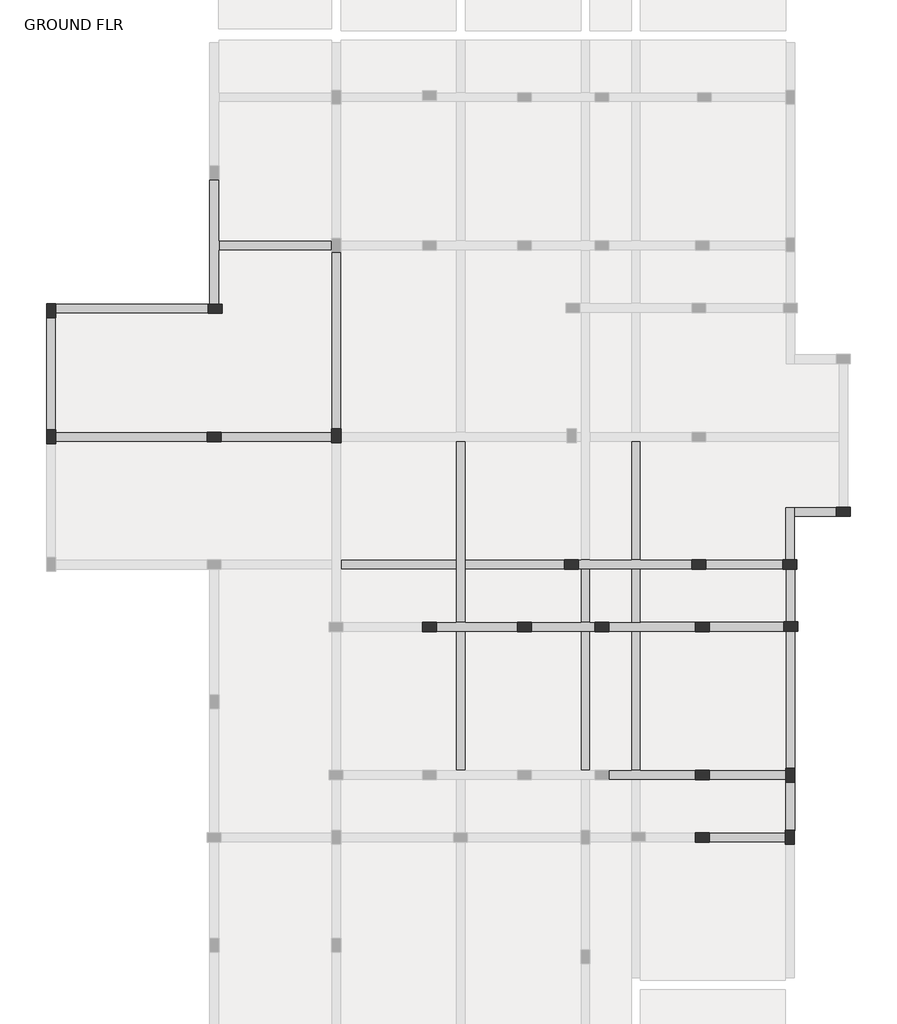
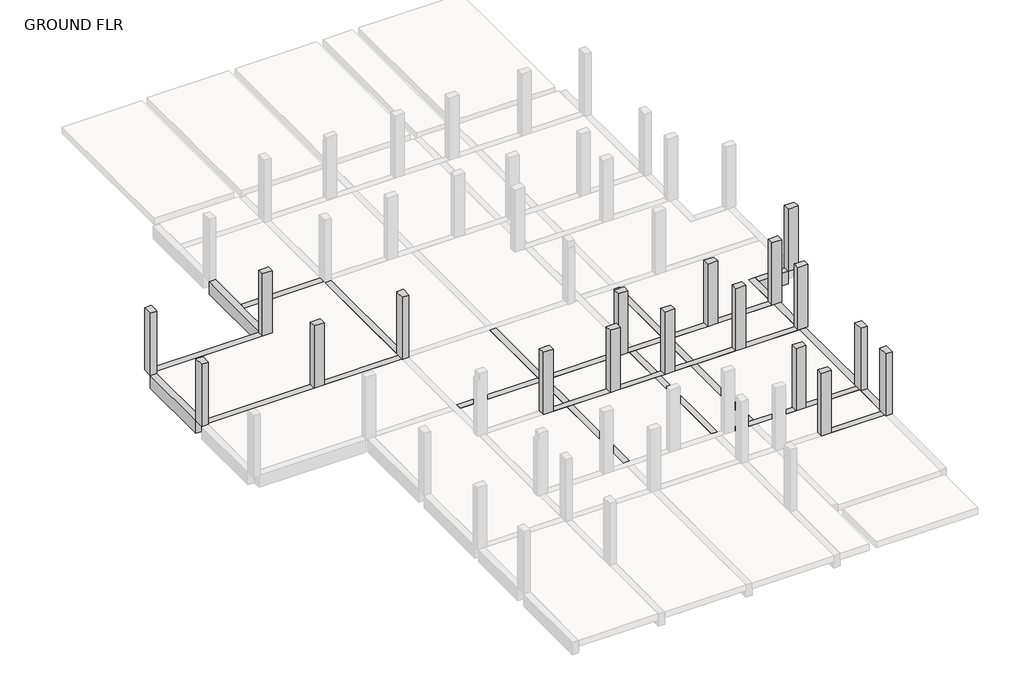
# One storey, part 3 of 5: 30 beams, 18 columns.
"""IFC4 building model written with IfcOpenShell, lengths in millimetres."""

from ifc_helpers import new_model, si_unit, frame, origin, place, context, project, spatial, polyline, outline, extrude, faceted_brep, element, save

model = new_model("IFC4")

# Units and contexts
model_context = context("Model", 3, world=origin())
ifc_project = project(units=[si_unit("LENGTHUNIT", "METRE", prefix="MILLI")], contexts=[model_context])

# Site, building, storey
site = spatial("IfcSite", under=ifc_project)
building = spatial("IfcBuilding", under=site)
storey = spatial("IfcBuildingStorey", under=building, Name="GROUND FLR", Elevation=0.0)

# Beams
placement = place(None, origin())
element("IfcBeam", 1, ObjectType="M_Concrete-Rectangular Beam : 300 x 600mm", at=placement, inside=storey, context=model_context, shape_type="Brep", body=[
    faceted_brep([(-5888.8105653, 9367.5252033, 0.0), (-5888.8105653, 5367.5252033, 0.0), (-5588.8105653, 5367.5252033, 0.0), (-5588.8105653, 7099.7076276, 0.0), (-5588.8105653, 7399.7076276, 0.0), (-5588.8105653, 9367.5252033, 0.0), (-5888.8105653, 9367.5252033, -600.0), (-5888.8105653, 5367.5252033, -600.0), (-5588.8105653, 9367.5252033, -600.0), (-5588.8105653, 7399.7076276, -600.0), (-5588.8105653, 7099.7076276, -600.0), (-5588.8105653, 5367.5252033, -600.0), (-5588.8105653, 9367.5252033, -300.0), (-5588.8105653, 5367.5252033, -300.0)], [[[0, 1, 2, 3, 4, 5]], [[1, 0, 6, 7]], [[7, 6, 8, 9, 10, 11]], [[11, 10, 9, 8, 12, 5, 4, 3, 2, 13]], [[8, 6, 0, 5, 12]], [[2, 1, 7, 11, 13]]]),
])
element("IfcBeam", 2, ObjectType="M_Concrete-Rectangular Beam : 300 x 600mm", at=placement, inside=storey, context=model_context, shape_type="Brep", body=[
    faceted_brep([(-5943.8105653, 5067.6057249, 0.0), (-5943.8105653, 5367.6057249, 0.0), (-10828.8105653, 5367.6057249, 0.0), (-10828.8105653, 5067.6057249, 0.0), (-5943.8105653, 5367.6057249, -600.0), (-10828.8105653, 5367.6057249, -600.0), (-5943.8105653, 5067.6057249, -600.0), (-10828.8105653, 5067.6057249, -600.0), (-10828.8105653, 5067.6057249, -300.0), (-5943.8105653, 5067.6057249, -300.0)], [[[0, 1, 2, 3]], [[1, 4, 5, 2]], [[4, 6, 7, 5]], [[0, 3, 8, 7, 6, 9]], [[6, 4, 1, 0, 9]], [[3, 2, 5, 7, 8]]]),
])
element("IfcBeam", 3, ObjectType="M_Concrete-Rectangular Beam : 300 x 600mm", at=placement, inside=storey, context=model_context, shape_type="SweptSolid", body=[
    extrude(outline(polyline([(-10828.8105653, 1326.1713929), (-11128.8105653, 1326.1713929), (-11128.8105653, 4932.6057249), (-10828.8105653, 4932.6057249), (-10828.8105653, 1326.1713929)])), frame((0.0, 0.0, -600.0), z_axis=(0.0, 0.0, 1.0), x_axis=(1.0, 0.0, 0.0)), (0.0, 0.0, 1.0), 600.0),
])
element("IfcBeam", 4, ObjectType="M_Concrete-Rectangular Beam : 300 x 600mm", at=placement, inside=storey, context=model_context, shape_type="SweptSolid", body=[
    extrude(outline(polyline([(12619.1163908, -9982.1078267), (12919.1163908, -9982.1078267), (12919.1163908, -11537.8970059), (12899.1163908, -11537.8970059), (12899.1163908, -11532.8970059), (12619.1163908, -11532.8970059), (12619.1163908, -9982.1078267)])), frame((0.0, 0.0, -600.0), z_axis=(0.0, 0.0, 1.0), x_axis=(1.0, 0.0, 0.0)), (0.0, 0.0, 1.0), 600.0),
])
element("IfcBeam", 5, ObjectType="M_Concrete-Rectangular Beam : 300 x 600mm", at=placement, inside=storey, context=model_context, shape_type="Brep", body=[
    faceted_brep([(12619.1163908, -5144.3229916, 0.0), (12919.1163908, -5144.3229916, 0.0), (12919.1163908, -5144.3229916, -600.0), (12619.1163908, -5144.3229916, -600.0), (12619.1163908, -5151.6229916, 0.0), (12619.1163908, -9532.1078267, 0.0), (12919.1163908, -9532.1078267, 0.0), (12919.1163908, -9532.1078267, -600.0), (12619.1163908, -9532.1078267, -600.0), (12619.1163908, -5151.6229916, -600.0), (12619.1163908, -9532.1078267, -300.0)], [[[0, 1, 2, 3]], [[1, 0, 4, 5, 6]], [[2, 1, 6, 7]], [[3, 2, 7, 8, 9]], [[0, 3, 9, 8, 10, 5, 4]], [[8, 7, 6, 5, 10]]]),
])
element("IfcBeam", 6, ObjectType="M_Concrete-Rectangular Beam : 300 x 600mm", at=placement, inside=storey, context=model_context, shape_type="Brep", body=[
    faceted_brep([(12619.1163908, -4818.9229916, -600.0), (12919.1163908, -4818.9229916, -600.0), (12919.1163908, -4818.9229916, 0.0), (12619.1163908, -4818.9229916, 0.0), (12619.1163908, -4818.9229916, -300.0), (12919.1163908, -3139.4535766, 0.0), (12619.1163908, -3139.4535766, 0.0), (12919.1163908, -3139.4535766, -600.0), (12619.1163908, -3139.4535766, -600.0), (12619.1163908, -3139.4535766, -300.0)], [[[0, 1, 2, 3, 4]], [[3, 2, 5, 6]], [[2, 1, 7, 5]], [[1, 0, 8, 7]], [[3, 6, 9, 8, 0, 4]], [[6, 5, 7, 8, 9]]]),
])
element("IfcBeam", 7, ObjectType="M_Concrete-Rectangular Beam : 300 x 600mm", at=placement, inside=storey, context=model_context, shape_type="Brep", body=[
    faceted_brep([(12599.1163908, -2839.4535766, 0.0), (12899.1163908, -2839.4535766, 0.0), (12899.1163908, -1448.8286071, 0.0), (12899.1163908, -1148.8286071, 0.0), (12599.1163908, -1148.8286071, 0.0), (12899.1163908, -2839.4535766, -600.0), (12899.1163908, -1448.8286071, -600.0), (12899.1163908, -1148.8286071, -600.0), (12899.1163908, -1148.8286071, -300.0), (12599.1163908, -2839.4535766, -600.0), (12599.1163908, -1148.8286071, -600.0), (12599.1163908, -1148.8286071, -300.0), (12599.1163908, -2839.4535766, -300.0)], [[[0, 1, 2, 3, 4]], [[1, 5, 6, 7, 8, 3, 2]], [[5, 9, 10, 7, 6]], [[0, 4, 11, 10, 9, 12]], [[9, 5, 1, 0, 12]], [[4, 3, 8, 7, 10, 11]]]),
])
element("IfcBeam", 8, ObjectType="M_Concrete-Rectangular Beam : 300 x 600mm", at=placement, inside=storey, context=model_context, shape_type="Brep", body=[
    faceted_brep([(14244.1163908, -1448.8286071, 0.0), (14244.1163908, -1148.8286071, 0.0), (12899.1163908, -1148.8286071, 0.0), (12899.1163908, -1448.8286071, 0.0), (14244.1163908, -1148.8286071, -300.0), (14244.1163908, -1148.8286071, -600.0), (12899.1163908, -1148.8286071, -600.0), (12899.1163908, -1148.8286071, -300.0), (14244.1163908, -1448.8286071, -600.0), (12899.1163908, -1448.8286071, -600.0)], [[[0, 1, 2, 3]], [[2, 1, 4, 5, 6, 7]], [[5, 8, 9, 6]], [[8, 0, 3, 9]], [[0, 8, 5, 4, 1]], [[3, 2, 7, 6, 9]]]),
])
element("IfcBeam", 9, ObjectType="M_Concrete-Rectangular Beam : 300 x 600mm", at=placement, inside=storey, context=model_context, shape_type="Brep", body=[
    faceted_brep([(-1671.7865686, 7024.7076276, 0.0), (-1971.7865686, 7024.7076276, 0.0), (-1971.7865686, 1366.1713929, 0.0), (-1671.7865686, 1366.1713929, 0.0), (-1971.7865686, 7024.7076276, -300.0), (-1971.7865686, 7024.7076276, -600.0), (-1971.7865686, 1366.1713929, -600.0), (-1971.7865686, 1366.1713929, -300.0), (-1671.7865686, 7024.7076276, -600.0), (-1671.7865686, 1366.1713929, -600.0), (-1671.7865686, 1366.1713929, -300.0), (-1671.7865686, 7024.7076276, -300.0)], [[[0, 1, 2, 3]], [[2, 1, 4, 5, 6, 7]], [[5, 8, 9, 6]], [[0, 3, 10, 9, 8, 11]], [[1, 0, 11, 8, 5, 4]], [[3, 2, 7, 6, 9, 10]]]),
])
element("IfcBeam", 10, ObjectType="M_Concrete-Rectangular Beam : 300 x 600mm", at=placement, inside=storey, context=model_context, shape_type="Brep", body=[
    faceted_brep([(-1971.7865686, 7099.7076276, 0.0), (-1971.7865686, 7399.7076276, 0.0), (-5588.8105653, 7399.7076276, 0.0), (-5588.8105653, 7099.7076276, 0.0), (-5588.8105653, 7099.7076276, -300.0), (-5588.8105653, 7099.7076276, -600.0), (-1971.7865686, 7099.7076276, -600.0), (-1971.7865686, 7099.7076276, -300.0), (-1971.7865686, 7399.7076276, -600.0), (-5588.8105653, 7399.7076276, -600.0), (-1971.7865686, 7399.7076276, -300.0), (-5588.8105653, 7399.7076276, -300.0)], [[[0, 1, 2, 3]], [[0, 3, 4, 5, 6, 7]], [[8, 6, 5, 9]], [[2, 1, 10, 8, 9, 11]], [[1, 0, 7, 6, 8, 10]], [[3, 2, 11, 9, 5, 4]]]),
])
element("IfcBeam", 11, ObjectType="M_Concrete-Rectangular Beam : 300 x 600mm", at=placement, inside=storey, context=model_context, shape_type="Brep", body=[
    faceted_brep([(-10828.8105653, 1251.1713929, 0.0), (-10828.8105653, 951.1713929, 0.0), (-5963.8105653, 951.1713929, 0.0), (-5963.8105653, 1251.1713929, 0.0), (-10828.8105653, 951.1713929, -300.0), (-10828.8105653, 951.1713929, -600.0), (-5963.8105653, 951.1713929, -600.0), (-5963.8105653, 951.1713929, -300.0), (-10828.8105653, 1251.1713929, -600.0), (-5963.8105653, 1251.1713929, -600.0), (-5963.8105653, 1251.1713929, -300.0), (-10828.8105653, 1251.1713929, -300.0)], [[[0, 1, 2, 3]], [[2, 1, 4, 5, 6, 7]], [[5, 8, 9, 6]], [[0, 3, 10, 9, 8, 11]], [[1, 0, 11, 8, 5, 4]], [[3, 2, 7, 6, 9, 10]]]),
])
element("IfcBeam", 12, ObjectType="M_Concrete-Rectangular Beam : 300 x 600mm", at=placement, inside=storey, context=model_context, shape_type="Brep", body=[
    faceted_brep([(-5513.8105653, 1251.1713929, 0.0), (-5513.8105653, 951.1713929, 0.0), (-1971.7865686, 951.1713929, 0.0), (-1971.7865686, 1251.1713929, 0.0), (-5513.8105653, 951.1713929, -300.0), (-5513.8105653, 951.1713929, -600.0), (-1971.7865686, 951.1713929, -600.0), (-1971.7865686, 951.1713929, -300.0), (-5513.8105653, 1251.1713929, -600.0), (-1971.7865686, 1251.1713929, -600.0), (-1971.7865686, 1251.1713929, -300.0), (-5513.8105653, 1251.1713929, -300.0)], [[[0, 1, 2, 3]], [[2, 1, 4, 5, 6, 7]], [[5, 8, 9, 6]], [[0, 3, 10, 9, 8, 11]], [[1, 0, 11, 8, 5, 4]], [[3, 2, 7, 6, 9, 10]]]),
])
element("IfcBeam", 13, ObjectType="M_Concrete-Rectangular Beam : 300 x 600mm", at=placement, inside=storey, context=model_context, shape_type="Brep", body=[
    faceted_brep([(9601.8679014, -3139.4535766, 0.0), (9601.8679014, -2839.4535766, 0.0), (7956.8679014, -2839.4535766, 0.0), (7656.8679014, -2839.4535766, 0.0), (6332.5248054, -2839.4535766, 0.0), (6032.5248054, -2839.4535766, 0.0), (5967.5248054, -2839.4535766, 0.0), (5967.5248054, -3139.4535766, 0.0), (6032.5248054, -3139.4535766, 0.0), (6332.5248054, -3139.4535766, 0.0), (7656.8679014, -3139.4535766, 0.0), (7956.8679014, -3139.4535766, 0.0), (5967.5248054, -3139.4535766, -600.0), (6032.5248054, -3139.4535766, -600.0), (6332.5248054, -3139.4535766, -600.0), (7656.8679014, -3139.4535766, -600.0), (7956.8679014, -3139.4535766, -600.0), (9601.8679014, -3139.4535766, -600.0), (9601.8679014, -3139.4535766, -300.0), (5967.5248054, -3139.4535766, -300.0), (9601.8679014, -2839.4535766, -600.0), (5967.5248054, -2839.4535766, -600.0), (6032.5248054, -2839.4535766, -600.0), (6332.5248054, -2839.4535766, -600.0), (7656.8679014, -2839.4535766, -600.0), (7956.8679014, -2839.4535766, -600.0), (5967.5248054, -2839.4535766, -300.0), (9601.8679014, -2839.4535766, -300.0)], [[[0, 1, 2, 3, 4, 5, 6, 7, 8, 9, 10, 11]], [[12, 13, 14, 15, 16, 17, 18, 0, 11, 10, 9, 8, 7, 19]], [[20, 17, 16, 15, 14, 13, 12, 21, 22, 23, 24, 25]], [[20, 25, 24, 23, 22, 21, 26, 6, 5, 4, 3, 2, 1, 27]], [[1, 0, 18, 17, 20, 27]], [[7, 6, 26, 21, 12, 19]]]),
])
element("IfcBeam", 14, ObjectType="M_Concrete-Rectangular Beam : 300 x 600mm", at=placement, inside=storey, context=model_context, shape_type="Brep", body=[
    faceted_brep([(12524.1163908, -3139.4535766, 0.0), (12524.1163908, -2839.4535766, 0.0), (10051.8679014, -2839.4535766, 0.0), (10051.8679014, -3139.4535766, 0.0), (10051.8679014, -3139.4535766, -300.0), (10051.8679014, -3139.4535766, -600.0), (12524.1163908, -3139.4535766, -600.0), (12524.1163908, -3139.4535766, -300.0), (12524.1163908, -2839.4535766, -600.0), (10051.8679014, -2839.4535766, -600.0), (12524.1163908, -2839.4535766, -300.0), (10051.8679014, -2839.4535766, -300.0)], [[[0, 1, 2, 3]], [[0, 3, 4, 5, 6, 7]], [[8, 6, 5, 9]], [[2, 1, 10, 8, 9, 11]], [[1, 0, 7, 6, 8, 10]], [[3, 2, 11, 9, 5, 4]]]),
])
element("IfcBeam", 15, ObjectType="M_Concrete-Rectangular Beam : 300 x 600mm", at=placement, inside=storey, context=model_context, shape_type="Brep", body=[
    faceted_brep([(1399.7296816, -4851.6229916, 0.0), (1399.7296816, -5151.6229916, 0.0), (2024.7296816, -5151.6229916, 0.0), (2324.7296816, -5151.6229916, 0.0), (3997.5248054, -5151.6229916, 0.0), (3997.5248054, -4851.6229916, 0.0), (2324.7296816, -4851.6229916, 0.0), (2024.7296816, -4851.6229916, 0.0), (1399.7296816, -5151.6229916, -600.0), (2024.7296816, -5151.6229916, -600.0), (2324.7296816, -5151.6229916, -600.0), (3997.5248054, -5151.6229916, -600.0), (3997.5248054, -5151.6229916, -300.0), (1399.7296816, -5151.6229916, -300.0), (1399.7296816, -4851.6229916, -600.0), (2024.7296816, -4851.6229916, -600.0), (2324.7296816, -4851.6229916, -600.0), (3997.5248054, -4851.6229916, -600.0), (1399.7296816, -4851.6229916, -300.0), (3997.5248054, -4851.6229916, -300.0)], [[[0, 1, 2, 3, 4, 5, 6, 7]], [[8, 9, 10, 11, 12, 4, 3, 2, 1, 13]], [[8, 14, 15, 16, 17, 11, 10, 9]], [[17, 16, 15, 14, 18, 0, 7, 6, 5, 19]], [[1, 0, 18, 14, 8, 13]], [[5, 4, 12, 11, 17, 19]]]),
])
element("IfcBeam", 16, ObjectType="M_Concrete-Rectangular Beam : 300 x 600mm", at=placement, inside=storey, context=model_context, shape_type="Brep", body=[
    faceted_brep([(4447.5248054, -4851.6229916, 0.0), (4447.5248054, -5151.6229916, 0.0), (6032.5248054, -5151.6229916, 0.0), (6332.5248054, -5151.6229916, 0.0), (6481.8679014, -5151.6229916, 0.0), (6481.8679014, -4851.6229916, 0.0), (6332.5248054, -4851.6229916, 0.0), (6032.5248054, -4851.6229916, 0.0), (4447.5248054, -5151.6229916, -600.0), (6032.5248054, -5151.6229916, -600.0), (6332.5248054, -5151.6229916, -600.0), (6481.8679014, -5151.6229916, -600.0), (6481.8679014, -5151.6229916, -300.0), (4447.5248054, -5151.6229916, -300.0), (4447.5248054, -4851.6229916, -600.0), (6032.5248054, -4851.6229916, -600.0), (6332.5248054, -4851.6229916, -600.0), (6481.8679014, -4851.6229916, -600.0), (4447.5248054, -4851.6229916, -300.0)], [[[0, 1, 2, 3, 4, 5, 6, 7]], [[8, 9, 10, 11, 12, 4, 3, 2, 1, 13]], [[8, 14, 15, 16, 17, 11, 10, 9]], [[17, 16, 15, 14, 18, 0, 7, 6, 5]], [[1, 0, 18, 14, 8, 13]], [[5, 4, 12, 11, 17]]]),
])
element("IfcBeam", 17, ObjectType="M_Concrete-Rectangular Beam : 300 x 600mm", at=placement, inside=storey, context=model_context, shape_type="Brep", body=[
    faceted_brep([(6931.8679014, -4851.6229916, 0.0), (6931.8679014, -5151.6229916, 0.0), (7656.8679014, -5151.6229916, 0.0), (7956.8679014, -5151.6229916, 0.0), (9721.8679014, -5151.6229916, 0.0), (9721.8679014, -4851.6229916, 0.0), (7956.8679014, -4851.6229916, 0.0), (7656.8679014, -4851.6229916, 0.0), (6931.8679014, -5151.6229916, -600.0), (7656.8679014, -5151.6229916, -600.0), (7956.8679014, -5151.6229916, -600.0), (9721.8679014, -5151.6229916, -600.0), (9721.8679014, -5151.6229916, -300.0), (6931.8679014, -5151.6229916, -300.0), (6931.8679014, -4851.6229916, -600.0), (7656.8679014, -4851.6229916, -600.0), (7956.8679014, -4851.6229916, -600.0), (9721.8679014, -4851.6229916, -600.0)], [[[0, 1, 2, 3, 4, 5, 6, 7]], [[8, 9, 10, 11, 12, 4, 3, 2, 1, 13]], [[8, 14, 15, 16, 17, 11, 10, 9]], [[14, 0, 7, 6, 5, 17, 16, 15]], [[1, 0, 14, 8, 13]], [[5, 4, 12, 11, 17]]]),
])
element("IfcBeam", 18, ObjectType="M_Concrete-Rectangular Beam : 300 x 600mm", at=placement, inside=storey, context=model_context, shape_type="Brep", body=[
    faceted_brep([(12599.1163908, -11907.8970059, 0.0), (12599.1163908, -11607.8970059, 0.0), (10171.8679014, -11607.8970059, 0.0), (10171.8679014, -11907.8970059, 0.0), (10171.8679014, -11907.8970059, -300.0), (10171.8679014, -11907.8970059, -600.0), (12599.1163908, -11907.8970059, -600.0), (12599.1163908, -11907.8970059, -300.0), (12599.1163908, -11607.8970059, -600.0), (10171.8679014, -11607.8970059, -600.0), (12599.1163908, -11607.8970059, -300.0), (10171.8679014, -11607.8970059, -300.0)], [[[0, 1, 2, 3]], [[0, 3, 4, 5, 6, 7]], [[8, 6, 5, 9]], [[2, 1, 10, 8, 9, 11]], [[1, 0, 7, 6, 8, 10]], [[3, 2, 11, 9, 5, 4]]]),
])
element("IfcBeam", 19, ObjectType="M_Concrete-Rectangular Beam : 300 x 600mm", at=placement, inside=storey, context=model_context, shape_type="Brep", body=[
    faceted_brep([(6931.8679014, -9607.1078267, 0.0), (6931.8679014, -9907.1078267, 0.0), (7656.8679014, -9907.1078267, 0.0), (7956.8679014, -9907.1078267, 0.0), (9721.8679014, -9907.1078267, 0.0), (9721.8679014, -9607.1078267, 0.0), (7956.8679014, -9607.1078267, 0.0), (7656.8679014, -9607.1078267, 0.0), (6931.8679014, -9907.1078267, -600.0), (7656.8679014, -9907.1078267, -600.0), (7956.8679014, -9907.1078267, -600.0), (9721.8679014, -9907.1078267, -600.0), (9721.8679014, -9907.1078267, -300.0), (6931.8679014, -9907.1078267, -300.0), (6931.8679014, -9607.1078267, -600.0), (7656.8679014, -9607.1078267, -600.0), (7956.8679014, -9607.1078267, -600.0), (9721.8679014, -9607.1078267, -600.0), (6931.8679014, -9607.1078267, -300.0), (9721.8679014, -9607.1078267, -300.0)], [[[0, 1, 2, 3, 4, 5, 6, 7]], [[8, 9, 10, 11, 12, 4, 3, 2, 1, 13]], [[8, 14, 15, 16, 17, 11, 10, 9]], [[17, 16, 15, 14, 18, 0, 7, 6, 5, 19]], [[1, 0, 18, 14, 8, 13]], [[5, 4, 12, 11, 17, 19]]]),
])
element("IfcBeam", 20, ObjectType="M_Concrete-Rectangular Beam : 300 x 600mm", at=placement, inside=storey, context=model_context, shape_type="Brep", body=[
    faceted_brep([(10171.8679014, -9607.1078267, 0.0), (10171.8679014, -9907.1078267, 0.0), (12599.1163908, -9907.1078267, 0.0), (12619.1163908, -9907.1078267, 0.0), (12619.1163908, -9607.1078267, 0.0), (10171.8679014, -9907.1078267, -600.0), (12619.1163908, -9907.1078267, -600.0), (10171.8679014, -9907.1078267, -300.0), (10171.8679014, -9607.1078267, -600.0), (12619.1163908, -9607.1078267, -600.0), (12619.1163908, -9607.1078267, -300.0), (10171.8679014, -9607.1078267, -300.0)], [[[0, 1, 2, 3, 4]], [[5, 6, 3, 2, 1, 7]], [[5, 8, 9, 6]], [[0, 4, 10, 9, 8, 11]], [[1, 0, 11, 8, 5, 7]], [[4, 3, 6, 9, 10]]]),
])
element("IfcBeam", 21, ObjectType="M_Concrete-Rectangular Beam : 300 x 600mm", at=placement, inside=storey, context=model_context, shape_type="Brep", body=[
    faceted_brep([(-1671.7865686, -2839.4535766, 0.0), (-1671.7865686, -3139.4535766, 0.0), (2024.7296816, -3139.4535766, 0.0), (2024.7296816, -2839.4535766, 0.0), (-1671.7865686, -3139.4535766, -300.0), (-1671.7865686, -3139.4535766, -600.0), (2024.7296816, -3139.4535766, -600.0), (2024.7296816, -3139.4535766, -300.0), (-1671.7865686, -2839.4535766, -600.0), (2024.7296816, -2839.4535766, -600.0), (2024.7296816, -2839.4535766, -300.0), (-1671.7865686, -2839.4535766, -300.0)], [[[0, 1, 2, 3]], [[2, 1, 4, 5, 6, 7]], [[5, 8, 9, 6]], [[0, 3, 10, 9, 8, 11]], [[1, 0, 11, 8, 5, 4]], [[3, 2, 7, 6, 9, 10]]]),
])
element("IfcBeam", 22, ObjectType="M_Concrete-Rectangular Beam : 300 x 600mm", at=placement, inside=storey, context=model_context, shape_type="Brep", body=[
    faceted_brep([(6332.5248054, -3139.4535766, 0.0), (6032.5248054, -3139.4535766, 0.0), (6032.5248054, -4851.6229916, 0.0), (6332.5248054, -4851.6229916, 0.0), (6032.5248054, -3139.4535766, -300.0), (6032.5248054, -3139.4535766, -600.0), (6032.5248054, -4851.6229916, -600.0), (6032.5248054, -4851.6229916, -300.0), (6332.5248054, -3139.4535766, -600.0), (6332.5248054, -4851.6229916, -600.0), (6332.5248054, -3139.4535766, -300.0), (6332.5248054, -4851.6229916, -300.0)], [[[0, 1, 2, 3]], [[2, 1, 4, 5, 6, 7]], [[5, 8, 9, 6]], [[8, 10, 0, 3, 11, 9]], [[1, 0, 10, 8, 5, 4]], [[3, 2, 7, 6, 9, 11]]]),
])
element("IfcBeam", 23, ObjectType="M_Concrete-Rectangular Beam : 300 x 600mm", at=placement, inside=storey, context=model_context, shape_type="Brep", body=[
    faceted_brep([(7956.8679014, -3139.4535766, 0.0), (7656.8679014, -3139.4535766, 0.0), (7656.8679014, -4851.6229916, 0.0), (7956.8679014, -4851.6229916, 0.0), (7956.8679014, -4831.6229916, 0.0), (7656.8679014, -3139.4535766, -300.0), (7656.8679014, -3139.4535766, -600.0), (7656.8679014, -4851.6229916, -600.0), (7656.8679014, -4851.6229916, -300.0), (7956.8679014, -3139.4535766, -600.0), (7956.8679014, -4851.6229916, -600.0), (7956.8679014, -3139.4535766, -300.0)], [[[0, 1, 2, 3, 4]], [[1, 5, 6, 7, 8, 2]], [[6, 9, 10, 7]], [[10, 9, 11, 0, 4, 3]], [[1, 0, 11, 9, 6, 5]], [[3, 2, 8, 7, 10]]]),
])
element("IfcBeam", 24, ObjectType="M_Concrete-Rectangular Beam : 300 x 600mm", at=placement, inside=storey, context=model_context, shape_type="Brep", body=[
    faceted_brep([(2324.7296816, -5151.6229916, 0.0), (2024.7296816, -5151.6229916, 0.0), (2024.7296816, -9607.1078267, 0.0), (2324.7296816, -9607.1078267, 0.0), (2024.7296816, -5151.6229916, -300.0), (2024.7296816, -5151.6229916, -600.0), (2024.7296816, -9607.1078267, -600.0), (2024.7296816, -9607.1078267, -300.0), (2324.7296816, -5151.6229916, -600.0), (2324.7296816, -9607.1078267, -600.0), (2324.7296816, -9607.1078267, -300.0), (2324.7296816, -5151.6229916, -300.0)], [[[0, 1, 2, 3]], [[2, 1, 4, 5, 6, 7]], [[5, 8, 9, 6]], [[0, 3, 10, 9, 8, 11]], [[1, 0, 11, 8, 5, 4]], [[3, 2, 7, 6, 9, 10]]]),
])
element("IfcBeam", 25, ObjectType="M_Concrete-Rectangular Beam : 300 x 600mm", at=placement, inside=storey, context=model_context, shape_type="Brep", body=[
    faceted_brep([(6332.5248054, -5151.6229916, 0.0), (6032.5248054, -5151.6229916, 0.0), (6032.5248054, -9607.1078267, 0.0), (6332.5248054, -9607.1078267, 0.0), (6032.5248054, -5151.6229916, -300.0), (6032.5248054, -5151.6229916, -600.0), (6032.5248054, -9607.1078267, -600.0), (6032.5248054, -9607.1078267, -300.0), (6332.5248054, -5151.6229916, -600.0), (6332.5248054, -9607.1078267, -600.0), (6332.5248054, -9607.1078267, -300.0), (6332.5248054, -5151.6229916, -300.0)], [[[0, 1, 2, 3]], [[2, 1, 4, 5, 6, 7]], [[5, 8, 9, 6]], [[0, 3, 10, 9, 8, 11]], [[1, 0, 11, 8, 5, 4]], [[3, 2, 7, 6, 9, 10]]]),
])
element("IfcBeam", 26, ObjectType="M_Concrete-Rectangular Beam : 300 x 600mm", at=placement, inside=storey, context=model_context, shape_type="Brep", body=[
    faceted_brep([(7956.8679014, -5151.6229916, 0.0), (7656.8679014, -5151.6229916, 0.0), (7656.8679014, -9607.1078267, 0.0), (7956.8679014, -9607.1078267, 0.0), (7656.8679014, -5151.6229916, -300.0), (7656.8679014, -5151.6229916, -600.0), (7656.8679014, -9607.1078267, -600.0), (7656.8679014, -9607.1078267, -300.0), (7956.8679014, -5151.6229916, -600.0), (7956.8679014, -9607.1078267, -600.0), (7956.8679014, -9607.1078267, -300.0), (7956.8679014, -5151.6229916, -300.0)], [[[0, 1, 2, 3]], [[2, 1, 4, 5, 6, 7]], [[5, 8, 9, 6]], [[0, 3, 10, 9, 8, 11]], [[1, 0, 11, 8, 5, 4]], [[3, 2, 7, 6, 9, 10]]]),
])
element("IfcBeam", 27, ObjectType="M_Concrete-Rectangular Beam : 300 x 600mm", at=placement, inside=storey, context=model_context, shape_type="Brep", body=[
    faceted_brep([(2024.7296816, -4851.6229916, 0.0), (2324.7296816, -4851.6229916, 0.0), (2324.7296816, -3139.4535766, 0.0), (2324.7296816, -2839.4535766, 0.0), (2324.7296816, 951.1713929, 0.0), (2024.7296816, 951.1713929, 0.0), (2024.7296816, -2839.4535766, 0.0), (2024.7296816, -3139.4535766, 0.0), (2024.7296816, 951.1713929, -600.0), (2024.7296816, -2839.4535766, -600.0), (2024.7296816, -3139.4535766, -600.0), (2024.7296816, -4851.6229916, -600.0), (2024.7296816, -4851.6229916, -300.0), (2024.7296816, 951.1713929, -300.0), (2324.7296816, -4851.6229916, -600.0), (2324.7296816, 951.1713929, -600.0), (2324.7296816, -2839.4535766, -600.0), (2324.7296816, -3139.4535766, -600.0), (2324.7296816, 951.1713929, -300.0), (2324.7296816, -4851.6229916, -300.0)], [[[0, 1, 2, 3, 4, 5, 6, 7]], [[8, 9, 10, 11, 12, 0, 7, 6, 5, 13]], [[14, 11, 10, 9, 8, 15, 16, 17]], [[14, 17, 16, 15, 18, 4, 3, 2, 1, 19]], [[1, 0, 12, 11, 14, 19]], [[5, 4, 18, 15, 8, 13]]]),
])
element("IfcBeam", 28, ObjectType="M_Concrete-Rectangular Beam : 300 x 600mm", at=placement, inside=storey, context=model_context, shape_type="Brep", body=[
    faceted_brep([(5517.5248054, -3139.4535766, 0.0), (5517.5248054, -2839.4535766, 0.0), (2324.7296816, -2839.4535766, 0.0), (2324.7296816, -3139.4535766, 0.0), (2324.7296816, -3139.4535766, -300.0), (2324.7296816, -3139.4535766, -600.0), (5517.5248054, -3139.4535766, -600.0), (5517.5248054, -3139.4535766, -300.0), (5517.5248054, -2839.4535766, -600.0), (2324.7296816, -2839.4535766, -600.0), (5517.5248054, -2839.4535766, -300.0), (2324.7296816, -2839.4535766, -300.0)], [[[0, 1, 2, 3]], [[0, 3, 4, 5, 6, 7]], [[8, 6, 5, 9]], [[2, 1, 10, 8, 9, 11]], [[1, 0, 7, 6, 8, 10]], [[3, 2, 11, 9, 5, 4]]]),
])
element("IfcBeam", 29, ObjectType="M_Concrete-Rectangular Beam : 300 x 600mm", at=placement, inside=storey, context=model_context, shape_type="Brep", body=[
    faceted_brep([(7656.8679014, -2839.4535766, 0.0), (7956.8679014, -2839.4535766, 0.0), (7956.8679014, 951.1713929, 0.0), (7656.8679014, 951.1713929, 0.0), (7656.8679014, 951.1713929, -300.0), (7656.8679014, 951.1713929, -600.0), (7656.8679014, -2839.4535766, -600.0), (7656.8679014, -2839.4535766, -300.0), (7956.8679014, -2839.4535766, -600.0), (7956.8679014, 951.1713929, -600.0), (7956.8679014, -2839.4535766, -300.0), (7956.8679014, 951.1713929, -300.0)], [[[0, 1, 2, 3]], [[0, 3, 4, 5, 6, 7]], [[8, 6, 5, 9]], [[2, 1, 10, 8, 9, 11]], [[1, 0, 7, 6, 8, 10]], [[3, 2, 11, 9, 5, 4]]]),
])
element("IfcBeam", 30, ObjectType="M_Concrete-Rectangular Beam : 300 x 600mm", at=placement, inside=storey, context=model_context, shape_type="Brep", body=[
    faceted_brep([(10171.8679014, -4851.6229916, 0.0), (10171.8679014, -5151.6229916, 0.0), (12619.1163908, -5151.6229916, 0.0), (12619.1163908, -5144.3229916, 0.0), (12919.1163908, -5144.3229916, 0.0), (12919.1163908, -5131.6229916, 0.0), (12564.1163908, -5131.6229916, 0.0), (12564.1163908, -4851.6229916, 0.0), (10171.8679014, -5151.6229916, -300.0), (10171.8679014, -5151.6229916, -600.0), (12619.1163908, -5151.6229916, -600.0), (12619.1163908, -5151.6229916, -300.0), (10171.8679014, -4851.6229916, -600.0), (12564.1163908, -4851.6229916, -600.0), (12564.1163908, -5131.6229916, -600.0), (12919.1163908, -5131.6229916, -600.0), (12919.1163908, -5144.3229916, -600.0), (12619.1163908, -5144.3229916, -600.0)], [[[0, 1, 2, 3, 4, 5, 6, 7]], [[2, 1, 8, 9, 10, 11]], [[9, 12, 13, 14, 15, 16, 17, 10]], [[12, 0, 7, 13]], [[4, 16, 15, 5]], [[1, 0, 12, 9, 8]], [[3, 17, 16, 4]], [[17, 3, 2, 11, 10]], [[14, 6, 5, 15]], [[6, 14, 13, 7]]]),
])

# Columns
element("IfcColumn", 31, ObjectType="M_Concrete-Rectangular-Column : 300 x 450mm", at=placement, inside=storey, context=model_context, shape_type="Brep", body=[
    faceted_brep([(-5943.8105653, 5367.6057249, 0.0), (-5493.8105653, 5367.6057249, 0.0), (-5493.8105653, 5067.6057249, 0.0), (-5943.8105653, 5067.6057249, 0.0), (-5943.8105653, 5367.6057249, 3000.0), (-5588.8105653, 5367.6057249, 3000.0), (-5493.8105653, 5367.6057249, 3000.0), (-5493.8105653, 5367.6057249, 2700.0), (-5493.8105653, 5067.6057249, 3000.0), (-5493.8105653, 5067.6057249, 2700.0), (-5943.8105653, 5067.6057249, 3000.0), (-5943.8105653, 5067.6057249, 2700.0)], [[[0, 1, 2, 3]], [[1, 0, 4, 5, 6, 7]], [[2, 1, 7, 6, 8, 9]], [[3, 2, 9, 8, 10, 11]], [[0, 3, 11, 10, 4]], [[8, 6, 5, 4, 10]]]),
])
element("IfcColumn", 32, ObjectType="M_Concrete-Rectangular-Column : 300 x 450mm", at=placement, inside=storey, context=model_context, shape_type="Brep", body=[
    faceted_brep([(-10828.8105653, 5382.6057249, 0.0), (-10828.8105653, 4932.6057249, 0.0), (-11128.8105653, 4932.6057249, 0.0), (-11128.8105653, 5382.6057249, 0.0), (-10828.8105653, 5382.6057249, 3000.0), (-10828.8105653, 5067.6057249, 3000.0), (-10828.8105653, 4932.6057249, 3000.0), (-11128.8105653, 4932.6057249, 3000.0), (-11128.8105653, 5382.6057249, 3000.0)], [[[0, 1, 2, 3]], [[4, 5, 6, 1, 0]], [[6, 7, 2, 1]], [[7, 8, 3, 2]], [[8, 4, 0, 3]], [[4, 8, 7, 6, 5]]]),
])
element("IfcColumn", 33, ObjectType="M_Concrete-Rectangular-Column : 300 x 450mm", at=placement, inside=storey, context=model_context, shape_type="Brep", body=[
    faceted_brep([(-11128.8105653, 876.1713929, 0.0), (-11128.8105653, 1326.1713929, 0.0), (-10828.8105653, 1326.1713929, 0.0), (-10828.8105653, 876.1713929, 0.0), (-11128.8105653, 876.1713929, 3000.0), (-11128.8105653, 1326.1713929, 3000.0), (-10828.8105653, 1326.1713929, 3000.0), (-10828.8105653, 1251.1713929, 3000.0), (-10828.8105653, 951.1713929, 3000.0), (-10828.8105653, 876.1713929, 3000.0)], [[[0, 1, 2, 3]], [[4, 5, 1, 0]], [[5, 6, 2, 1]], [[6, 7, 8, 9, 3, 2]], [[9, 4, 0, 3]], [[4, 9, 8, 7, 6, 5]]]),
])
element("IfcColumn", 34, ObjectType="M_Concrete-Rectangular-Column : 300 x 450mm", at=placement, inside=storey, context=model_context, shape_type="Brep", body=[
    faceted_brep([(-5513.8105653, 951.1713929, 0.0), (-5963.8105653, 951.1713929, 0.0), (-5963.8105653, 1251.1713929, 0.0), (-5513.8105653, 1251.1713929, 0.0), (-5513.8105653, 951.1713929, 2700.0), (-5513.8105653, 951.1713929, 3000.0), (-5963.8105653, 951.1713929, 3000.0), (-5963.8105653, 951.1713929, 2700.0), (-5963.8105653, 1251.1713929, 3000.0), (-5963.8105653, 1251.1713929, 2700.0), (-5513.8105653, 1251.1713929, 3000.0), (-5513.8105653, 1251.1713929, 2700.0)], [[[0, 1, 2, 3]], [[1, 0, 4, 5, 6, 7]], [[2, 1, 7, 6, 8, 9]], [[3, 2, 9, 8, 10, 11]], [[0, 3, 11, 10, 5, 4]], [[6, 5, 10, 8]]]),
])
element("IfcColumn", 35, ObjectType="M_Concrete-Rectangular-Column : 300 x 450mm", at=placement, inside=storey, context=model_context, shape_type="Brep", body=[
    faceted_brep([(-1671.7865686, 1366.1713929, 0.0), (-1671.7865686, 916.1713929, 0.0), (-1971.7865686, 916.1713929, 0.0), (-1971.7865686, 1366.1713929, 0.0), (-1671.7865686, 1366.1713929, 2700.0), (-1671.7865686, 1366.1713929, 3000.0), (-1671.7865686, 1251.1713929, 3000.0), (-1671.7865686, 951.1713929, 3000.0), (-1671.7865686, 916.1713929, 3000.0), (-1671.7865686, 916.1713929, 2700.0), (-1971.7865686, 916.1713929, 3000.0), (-1971.7865686, 916.1713929, 2700.0), (-1971.7865686, 951.1713929, 3000.0), (-1971.7865686, 1251.1713929, 3000.0), (-1971.7865686, 1366.1713929, 3000.0), (-1971.7865686, 1366.1713929, 2700.0)], [[[0, 1, 2, 3]], [[1, 0, 4, 5, 6, 7, 8, 9]], [[2, 1, 9, 8, 10, 11]], [[3, 2, 11, 10, 12, 13, 14, 15]], [[0, 3, 15, 14, 5, 4]], [[10, 8, 7, 6, 5, 14, 13, 12]]]),
])
element("IfcColumn", 36, ObjectType="M_Concrete-Rectangular-Column : 300 x 450mm", at=placement, inside=storey, context=model_context, shape_type="Brep", body=[
    faceted_brep([(14244.1163908, -1148.8286071, 0.0), (14694.1163908, -1148.8286071, 0.0), (14694.1163908, -1448.8286071, 0.0), (14244.1163908, -1448.8286071, 0.0), (14244.1163908, -1148.8286071, 2700.0), (14244.1163908, -1148.8286071, 3000.0), (14319.1163908, -1148.8286071, 3000.0), (14694.1163908, -1148.8286071, 3000.0), (14694.1163908, -1448.8286071, 3000.0), (14244.1163908, -1448.8286071, 3000.0)], [[[0, 1, 2, 3]], [[1, 0, 4, 5, 6, 7]], [[2, 1, 7, 8]], [[3, 2, 8, 9]], [[0, 3, 9, 5, 4]], [[8, 7, 6, 5, 9]]]),
])
element("IfcColumn", 37, ObjectType="M_Concrete-Rectangular-Column : 300 x 450mm", at=placement, inside=storey, context=model_context, shape_type="Brep", body=[
    faceted_brep([(12524.1163908, -2839.4535766, 0.0), (12974.1163908, -2839.4535766, 0.0), (12974.1163908, -3139.4535766, 0.0), (12524.1163908, -3139.4535766, 0.0), (12524.1163908, -2839.4535766, 2700.0), (12524.1163908, -2839.4535766, 3000.0), (12599.1163908, -2839.4535766, 3000.0), (12974.1163908, -2839.4535766, 3000.0), (12974.1163908, -3139.4535766, 3000.0), (12619.1163908, -3139.4535766, 3000.0), (12524.1163908, -3139.4535766, 3000.0), (12524.1163908, -3139.4535766, 2700.0)], [[[0, 1, 2, 3]], [[1, 0, 4, 5, 6, 7]], [[2, 1, 7, 8]], [[3, 2, 8, 9, 10, 11]], [[0, 3, 11, 10, 5, 4]], [[8, 7, 6, 5, 10, 9]]]),
])
element("IfcColumn", 38, ObjectType="M_Concrete-Rectangular-Column : 300 x 450mm", at=placement, inside=storey, context=model_context, shape_type="Brep", body=[
    faceted_brep([(9601.8679014, -2839.4535766, 0.0), (10051.8679014, -2839.4535766, 0.0), (10051.8679014, -3139.4535766, 0.0), (9601.8679014, -3139.4535766, 0.0), (9601.8679014, -2839.4535766, 2700.0), (9601.8679014, -2839.4535766, 3000.0), (10051.8679014, -2839.4535766, 3000.0), (10051.8679014, -2839.4535766, 2700.0), (10051.8679014, -3139.4535766, 3000.0), (10051.8679014, -3139.4535766, 2700.0), (9601.8679014, -3139.4535766, 3000.0), (9601.8679014, -3139.4535766, 2700.0)], [[[0, 1, 2, 3]], [[1, 0, 4, 5, 6, 7]], [[2, 1, 7, 6, 8, 9]], [[3, 2, 9, 8, 10, 11]], [[0, 3, 11, 10, 5, 4]], [[6, 5, 10, 8]]]),
])
element("IfcColumn", 39, ObjectType="M_Concrete-Rectangular-Column : 300 x 450mm", at=placement, inside=storey, context=model_context, shape_type="Brep", body=[
    faceted_brep([(5517.5248054, -2839.4535766, 0.0), (5967.5248054, -2839.4535766, 0.0), (5967.5248054, -3139.4535766, 0.0), (5517.5248054, -3139.4535766, 0.0), (5517.5248054, -2839.4535766, 2700.0), (5517.5248054, -2839.4535766, 3000.0), (5967.5248054, -2839.4535766, 3000.0), (5967.5248054, -2839.4535766, 2700.0), (5967.5248054, -3139.4535766, 3000.0), (5967.5248054, -3139.4535766, 2700.0), (5517.5248054, -3139.4535766, 3000.0), (5517.5248054, -3139.4535766, 2700.0)], [[[0, 1, 2, 3]], [[1, 0, 4, 5, 6, 7]], [[2, 1, 7, 6, 8, 9]], [[3, 2, 9, 8, 10, 11]], [[0, 3, 11, 10, 5, 4]], [[6, 5, 10, 8]]]),
])
element("IfcColumn", 40, ObjectType="M_Concrete-Rectangular-Column : 300 x 450mm", at=placement, inside=storey, context=model_context, shape_type="Brep", body=[
    faceted_brep([(1399.7296816, -5151.6229916, 0.0), (949.7296816, -5151.6229916, 0.0), (949.7296816, -4851.6229916, 0.0), (1399.7296816, -4851.6229916, 0.0), (1399.7296816, -5151.6229916, 2700.0), (1399.7296816, -5151.6229916, 3000.0), (949.7296816, -5151.6229916, 3000.0), (949.7296816, -5151.6229916, 2700.0), (949.7296816, -4851.6229916, 3000.0), (949.7296816, -4851.6229916, 2700.0), (1399.7296816, -4851.6229916, 3000.0), (1399.7296816, -4851.6229916, 2700.0)], [[[0, 1, 2, 3]], [[1, 0, 4, 5, 6, 7]], [[2, 1, 7, 6, 8, 9]], [[3, 2, 9, 8, 10, 11]], [[0, 3, 11, 10, 5, 4]], [[6, 5, 10, 8]]]),
])
element("IfcColumn", 41, ObjectType="M_Concrete-Rectangular-Column : 300 x 450mm", at=placement, inside=storey, context=model_context, shape_type="Brep", body=[
    faceted_brep([(4447.5248054, -5151.6229916, 0.0), (3997.5248054, -5151.6229916, 0.0), (3997.5248054, -4851.6229916, 0.0), (4447.5248054, -4851.6229916, 0.0), (4447.5248054, -5151.6229916, 2700.0), (4447.5248054, -5151.6229916, 3000.0), (3997.5248054, -5151.6229916, 3000.0), (3997.5248054, -5151.6229916, 2700.0), (3997.5248054, -4851.6229916, 3000.0), (3997.5248054, -4851.6229916, 2700.0), (4447.5248054, -4851.6229916, 3000.0), (4447.5248054, -4851.6229916, 2700.0)], [[[0, 1, 2, 3]], [[1, 0, 4, 5, 6, 7]], [[2, 1, 7, 6, 8, 9]], [[3, 2, 9, 8, 10, 11]], [[0, 3, 11, 10, 5, 4]], [[6, 5, 10, 8]]]),
])
element("IfcColumn", 42, ObjectType="M_Concrete-Rectangular-Column : 300 x 450mm", at=placement, inside=storey, context=model_context, shape_type="Brep", body=[
    faceted_brep([(6931.8679014, -5151.6229916, 0.0), (6481.8679014, -5151.6229916, 0.0), (6481.8679014, -4851.6229916, 0.0), (6931.8679014, -4851.6229916, 0.0), (6931.8679014, -5151.6229916, 2700.0), (6931.8679014, -5151.6229916, 3000.0), (6481.8679014, -5151.6229916, 3000.0), (6481.8679014, -5151.6229916, 2700.0), (6481.8679014, -4851.6229916, 3000.0), (6931.8679014, -4851.6229916, 3000.0)], [[[0, 1, 2, 3]], [[1, 0, 4, 5, 6, 7]], [[2, 1, 7, 6, 8]], [[3, 2, 8, 9]], [[0, 3, 9, 5, 4]], [[6, 5, 9, 8]]]),
])
element("IfcColumn", 43, ObjectType="M_Concrete-Rectangular-Column : 300 x 450mm", at=placement, inside=storey, context=model_context, shape_type="Brep", body=[
    faceted_brep([(10171.8679014, -5151.6229916, 0.0), (9721.8679014, -5151.6229916, 0.0), (9721.8679014, -4851.6229916, 0.0), (10171.8679014, -4851.6229916, 0.0), (10171.8679014, -5151.6229916, 2700.0), (10171.8679014, -5151.6229916, 3000.0), (9721.8679014, -5151.6229916, 3000.0), (9721.8679014, -5151.6229916, 2700.0), (9721.8679014, -4851.6229916, 3000.0), (10171.8679014, -4851.6229916, 3000.0)], [[[0, 1, 2, 3]], [[1, 0, 4, 5, 6, 7]], [[2, 1, 7, 6, 8]], [[3, 2, 8, 9]], [[0, 3, 9, 5, 4]], [[6, 5, 9, 8]]]),
])
element("IfcColumn", 44, ObjectType="M_Concrete-Rectangular-Column : 300 x 450mm", at=placement, inside=storey, context=model_context, shape_type="Brep", body=[
    faceted_brep([(13014.1163908, -5131.6229916, 0.0), (12564.1163908, -5131.6229916, 0.0), (12564.1163908, -4831.6229916, 0.0), (13014.1163908, -4831.6229916, 0.0), (13014.1163908, -5131.6229916, 3000.0), (12564.1163908, -5131.6229916, 3000.0), (12564.1163908, -4831.6229916, 3000.0), (12564.1163908, -4831.6229916, 2700.0), (12619.1163908, -4831.6229916, 3000.0), (13014.1163908, -4831.6229916, 3000.0)], [[[0, 1, 2, 3]], [[1, 0, 4, 5]], [[2, 1, 5, 6, 7]], [[3, 2, 7, 6, 8, 9]], [[0, 3, 9, 4]], [[5, 4, 9, 8, 6]]]),
])
element("IfcColumn", 45, ObjectType="M_Concrete-Rectangular-Column : 300 x 450mm", at=placement, inside=storey, context=model_context, shape_type="Brep", body=[
    faceted_brep([(10171.8679014, -9907.1078267, 0.0), (9721.8679014, -9907.1078267, 0.0), (9721.8679014, -9607.1078267, 0.0), (10171.8679014, -9607.1078267, 0.0), (10171.8679014, -9907.1078267, 2700.0), (10171.8679014, -9907.1078267, 3000.0), (9721.8679014, -9907.1078267, 3000.0), (9721.8679014, -9907.1078267, 2700.0), (9721.8679014, -9607.1078267, 3000.0), (9721.8679014, -9607.1078267, 2700.0), (10171.8679014, -9607.1078267, 3000.0), (10171.8679014, -9607.1078267, 2700.0)], [[[0, 1, 2, 3]], [[1, 0, 4, 5, 6, 7]], [[2, 1, 7, 6, 8, 9]], [[3, 2, 9, 8, 10, 11]], [[0, 3, 11, 10, 5, 4]], [[6, 5, 10, 8]]]),
])
element("IfcColumn", 46, ObjectType="M_Concrete-Rectangular-Column : 300 x 450mm", at=placement, inside=storey, context=model_context, shape_type="Brep", body=[
    faceted_brep([(12919.1163908, -9532.1078267, 0.0), (12919.1163908, -9982.1078267, 0.0), (12619.1163908, -9982.1078267, 0.0), (12619.1163908, -9532.1078267, 0.0), (12919.1163908, -9532.1078267, 3000.0), (12919.1163908, -9982.1078267, 3000.0), (12619.1163908, -9982.1078267, 3000.0), (12619.1163908, -9607.1078267, 3000.0), (12619.1163908, -9532.1078267, 3000.0), (12619.1163908, -9532.1078267, 2700.0)], [[[0, 1, 2, 3]], [[1, 0, 4, 5]], [[2, 1, 5, 6]], [[3, 2, 6, 7, 8, 9]], [[0, 3, 9, 8, 4]], [[5, 4, 8, 7, 6]]]),
])
element("IfcColumn", 47, ObjectType="M_Concrete-Rectangular-Column : 300 x 450mm", at=placement, inside=storey, context=model_context, shape_type="Brep", body=[
    faceted_brep([(12899.1163908, -11532.8970059, 0.0), (12899.1163908, -11982.8970059, 0.0), (12599.1163908, -11982.8970059, 0.0), (12599.1163908, -11532.8970059, 0.0), (12899.1163908, -11532.8970059, 3000.0), (12899.1163908, -11982.8970059, 3000.0), (12599.1163908, -11982.8970059, 3000.0), (12599.1163908, -11982.8970059, 2700.0), (12599.1163908, -11907.8970059, 3000.0), (12599.1163908, -11607.8970059, 3000.0), (12599.1163908, -11532.8970059, 3000.0), (12599.1163908, -11532.8970059, 2700.0)], [[[0, 1, 2, 3]], [[1, 0, 4, 5]], [[2, 1, 5, 6, 7]], [[3, 2, 7, 6, 8, 9, 10, 11]], [[0, 3, 11, 10, 4]], [[5, 4, 10, 9, 8, 6]]]),
])
element("IfcColumn", 48, ObjectType="M_Concrete-Rectangular-Column : 300 x 450mm", at=placement, inside=storey, context=model_context, shape_type="Brep", body=[
    faceted_brep([(9721.8679014, -11607.8970059, 0.0), (10171.8679014, -11607.8970059, 0.0), (10171.8679014, -11907.8970059, 0.0), (9721.8679014, -11907.8970059, 0.0), (9721.8679014, -11607.8970059, 2700.0), (9721.8679014, -11607.8970059, 3000.0), (10171.8679014, -11607.8970059, 3000.0), (10171.8679014, -11607.8970059, 2700.0), (10171.8679014, -11907.8970059, 3000.0), (10171.8679014, -11907.8970059, 2700.0), (9721.8679014, -11907.8970059, 3000.0), (9721.8679014, -11907.8970059, 2700.0)], [[[0, 1, 2, 3]], [[1, 0, 4, 5, 6, 7]], [[2, 1, 7, 6, 8, 9]], [[3, 2, 9, 8, 10, 11]], [[0, 3, 11, 10, 5, 4]], [[6, 5, 10, 8]]]),
])

save(model, "model.ifc")

# Revit data of these elements
# Type "M_Concrete-Rectangular Beam : 300 x 600mm"
#   Length [instance default] = 1524 mm
#   b = 300 mm
#   h = 600 mm
#   Structural Material [instance default] = Concrete, Cast-in-Place gray
#   Assembly Code = ""
# Type "M_Concrete-Rectangular-Column : 300 x 450mm"
#   b = 300 mm
#   h = 450 mm
#   Structural Material [instance default] = Concrete, Cast-in-Place gray
# Elements 1, 2, 3, 4, 5, 6, 7, 8, 9, 10, 11, 12, 13, 14, 15, 16, 17, 18, 19, 20, 30 (IfcBeam, "M_Concrete-Rectangular Beam : 300 x 600mm")
#   Structural Material = Concrete, Cast-in-Place gray
#   Phase Created = New Construction
#   Materials on its faces: "Concrete, Cast-in-Place gray"
# Elements 21, 28 (IfcBeam, "M_Concrete-Rectangular Beam : 300 x 600mm")
#   IfcGUID = "1qukP20bvFNgU5pJ1DIAvo"
#   Phase Created = New Construction
#   Materials on its faces: "Concrete, Cast-in-Place gray"
# Elements 22, 25 (IfcBeam, "M_Concrete-Rectangular Beam : 300 x 600mm")
#   IfcGUID = "1qukP20bvFNgU5pJ1DIAuc"
#   Phase Created = New Construction
#   Materials on its faces: "Concrete, Cast-in-Place gray"
# Elements 23, 26, 29 (IfcBeam, "M_Concrete-Rectangular Beam : 300 x 600mm")
#   IfcGUID = "1qukP20bvFNgU5pJ1DIAvT"
#   Phase Created = New Construction
#   Materials on its faces: "Concrete, Cast-in-Place gray"
# Elements 24, 27 (IfcBeam, "M_Concrete-Rectangular Beam : 300 x 600mm")
#   IfcGUID = "1qukP20bvFNgU5pJ1DIAuk"
#   Phase Created = New Construction
#   Materials on its faces: "Concrete, Cast-in-Place gray"
# Elements 31, 32, 33, 34, 35, 36, 37, 38, 39, 40, 41, 42, 43, 44, 45, 46, 47, 48 (IfcColumn, "M_Concrete-Rectangular-Column : 300 x 450mm")
#   Structural Material = Concrete, Cast-in-Place gray
#   Phase Created = New Construction
#   Materials on its faces: "Concrete, Cast-in-Place gray"
# Materials
#   "Concrete, Cast-in-Place gray": class "Concrete", colour RGB 192 192 192, transparency 0, Description = "Cast-in-place concrete", Cost = 0
